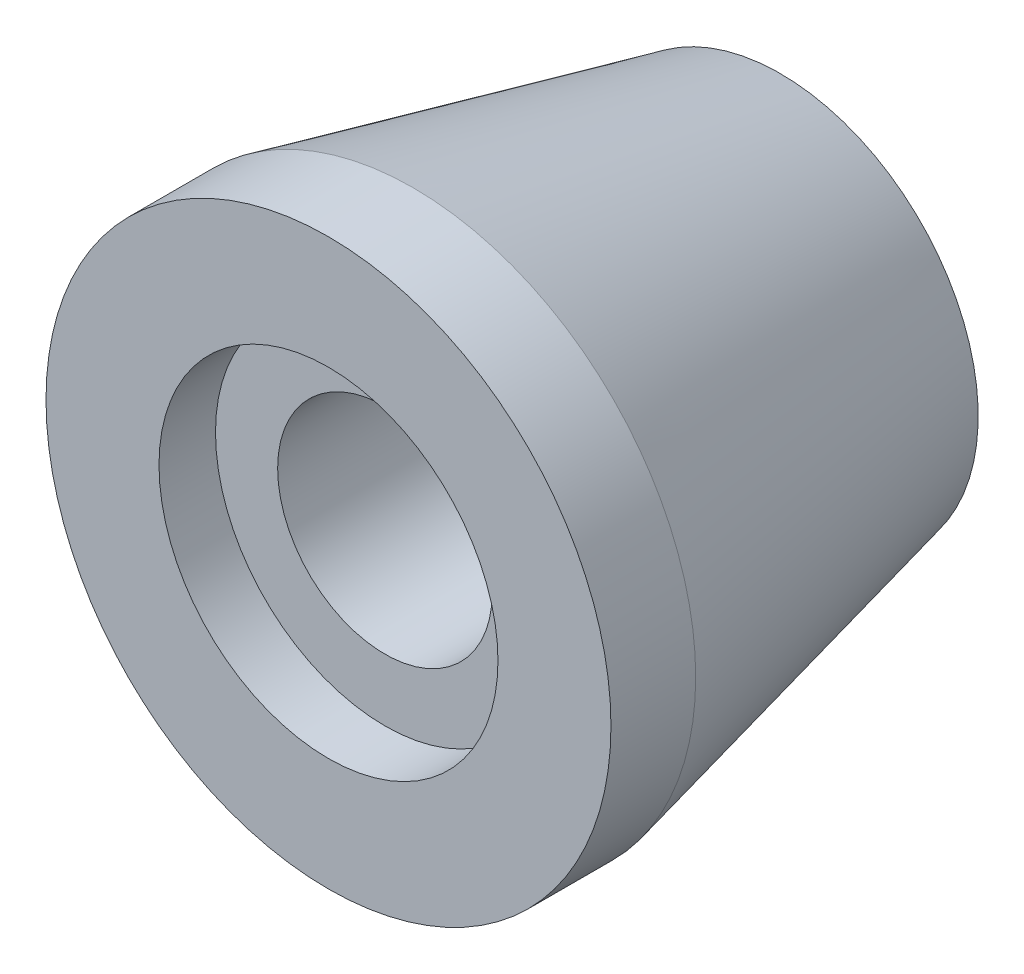
from build123d import *


with BuildPart() as part:
    # Bushing Profile Sketch → Bushing Body Revolve (revolve)
    with BuildSketch(Plane(origin=(0, 0, 0), x_dir=(0, 0, -1), z_dir=(1, 0, 0)), mode=Mode.PRIVATE) as bushing_body_revolve_sk:
        Polygon((0, 3.8), (-14, 3.8), (-14, 6), (-16, 6), (-16, 10), (-13, 10), (0, 7), align=None)
    revolve(bushing_body_revolve_sk.sketch.rotate(Axis((0, 0, 0), (0, 0, 1)), 90), axis=Axis((0, 0, 0), (0, 0, 1)))


solid = part.part
